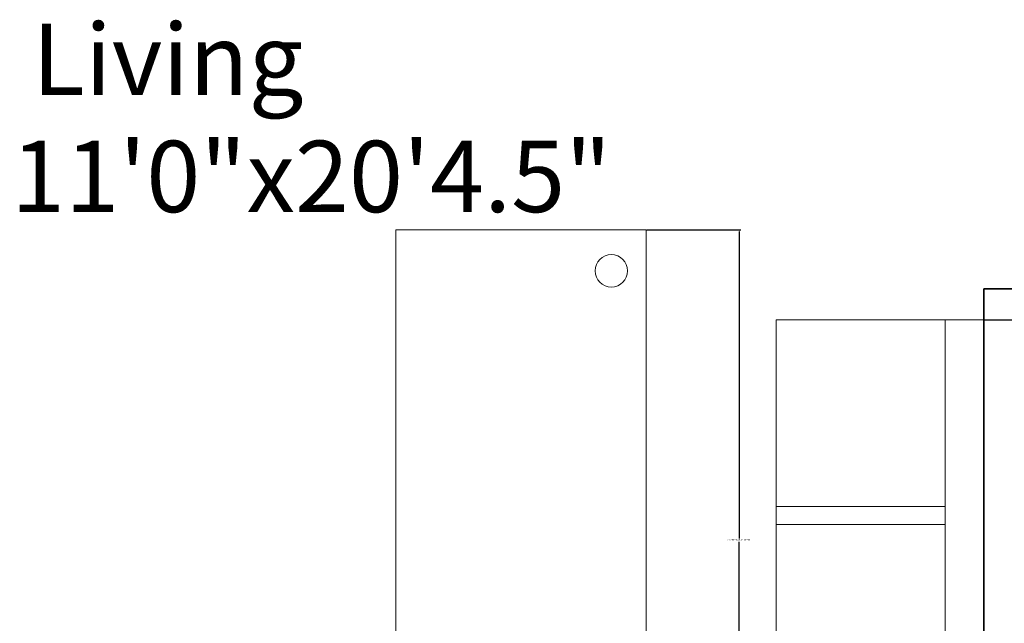
# Model space of a CAD drawing. Units: inches. Extents: x 108 to 613, y 1573 to 2319.
# Tile 7 of 11: x 325 to 434, y 2055 to 2122. Entities that reach past the tile are written whole.
import ezdxf

# ---------------------------------------------------------------- set-up
doc = ezdxf.new("R2010")
doc.units = ezdxf.units.IN
for name, color, linetype, lineweight in [('A-ANNO-DIMS', 2, 'Continuous', 18), ('A-AREA-IDEN', 3, 'Continuous', 18), ('furniture', 2, 'Continuous', 18), ('wall', 6, 'Continuous', 35)]:
    doc.layers.add(name, color=color, linetype=linetype, lineweight=lineweight)
doc.styles.get("Standard").update_dxf_attribs({"font": 'arial.ttf'})
doc.dimstyles.get("Standard").update_dxf_attribs({"dimtxt": 0.18, "dimasz": 0.18, "dimexe": 0.18, "dimexo": 0.0625, "dimgap": 0.09, "dimtad": 0, "dimtih": 1, "dimtoh": 1, "dimdec": 4, "dimzin": 0, "dimdsep": 46, "dimtxsty": 'Standard', "dimcen": 0.09, "dimadec": 0, "dimazin": 0, "dimtfac": 1, "dimtdec": 4, "dimtofl": 0, "dimtmove": 0, "dimatfit": 3, "dimfxl": 1, "dimtolj": 1, "dimtzin": 0, "dimarcsym": 0})

# ---------------------------------------------------------------- blocks, each defined once
blk = doc.blocks.new('COFFEE-TABLE')
blk.add_lwpolyline([(0, 68.46), (27.63, 68.46), (27.63, 0), (0, 0)], close=True)
for centre, radius in [((23.79, 63.93), 1.79), ((3.47, 4.05), 1.83)]:
    blk.add_circle(centre, radius)
blk = doc.blocks.new('SOFA-3-SEAT')
for p, q in [((18.7, 63.66), (18.7, 0)), ((0.03, 43.08), (18.7, 43.08)), ((0.03, 41.08), (18.7, 41.08)), ((0.03, 20.17), (18.7, 19.89)), ((0, 18.17), (18.7, 17.89))]:
    blk.add_line(p, q)
blk.add_lwpolyline([(0.03, 63.66), (22.97, 63.66), (22.97, 0), (0.03, 0)], close=True)
blk = doc.blocks.new('*D29')
at = {"layer": 'A-ANNO-DIMS', "color": 0, "lineweight": -2, "transparency": 16777216}
for p, q in [((394.08, 2098.63), (404.46, 2098.63)), ((404.28, 2098.45), (404.28, 2064.59)), ((404.28, 2030.36), (404.28, 2064.22)), ((394.08, 2030.18), (404.46, 2030.18))]:
    blk.add_line(p, q, dxfattribs=at)
at = {"layer": 'A-ANNO-DIMS', "color": 0, "transparency": 16777216}
for points in [[(404.25, 2098.45), (404.31, 2098.45), (404.28, 2098.63)], [(404.25, 2030.36), (404.31, 2030.36), (404.28, 2030.18)]]:
    blk.add_solid(points, dxfattribs=at)
at = {"layer": 'Defpoints', "color": 0, "transparency": 16777216}
for p in [(394.01, 2098.63), (404.28, 2098.63), (394.01, 2030.18)]:
    blk.add_point(p, dxfattribs=at)
at = {"layer": 'A-ANNO-DIMS', "color": 0, "transparency": 16777216, "insert": (404.28, 2064.41), "char_height": 0.18, "attachment_point": 5}
blk.add_mtext('\\A1;COFFEE TABLE 68 TYP.', dxfattribs=at)
blk = doc.blocks.new('*D31')
at = {"layer": 'A-ANNO-DIMS', "color": 0, "lineweight": -2, "transparency": 16777216}
for p, q in [((431.34, 2088.69), (441, 2088.69)), ((440.82, 2088.51), (440.82, 2057.05)), ((440.82, 2025.21), (440.82, 2056.68)), ((431.34, 2025.03), (441, 2025.03))]:
    blk.add_line(p, q, dxfattribs=at)
at = {"layer": 'A-ANNO-DIMS', "color": 0, "transparency": 16777216}
for points in [[(440.79, 2088.51), (440.85, 2088.51), (440.82, 2088.69)], [(440.79, 2025.21), (440.85, 2025.21), (440.82, 2025.03)]]:
    blk.add_solid(points, dxfattribs=at)
at = {"layer": 'Defpoints', "color": 0, "transparency": 16777216}
for p in [(431.28, 2088.69), (440.82, 2088.69), (431.28, 2025.03)]:
    blk.add_point(p, dxfattribs=at)
at = {"layer": 'A-ANNO-DIMS', "color": 0, "transparency": 16777216, "insert": (440.82, 2056.86), "char_height": 0.18, "attachment_point": 5}
blk.add_mtext('\\A1;3-SEAT SOFA 64 TYP.', dxfattribs=at)

msp = doc.modelspace()

# ---------------------------------------------------------------- linework, layer by layer
at = {"layer": 'wall'}
for q in [(435.7753, 2092.1125), (431.2753, 1997.6125)]:
    msp.add_line((431.2753, 2092.1125), q, dxfattribs=at)

# ---------------------------------------------------------------- block references
at = {"layer": 'furniture'}
for name, p in [('COFFEE-TABLE', (366.385, 2030.176)), ('SOFA-3-SEAT', (408.31, 2025.033))]:
    msp.add_blockref(name, p, dxfattribs=at)

# ---------------------------------------------------------------- texts
at = {"layer": 'A-AREA-IDEN'}
for s, height, p in [('Living', 7.87346, (326.2616, 2113.4914)), ('11\'0"x20\'4.5"', 7.873465, (323.9532, 2100.5856))]:
    msp.add_text(s, height=height, dxfattribs=at).set_placement(p)

# ---------------------------------------------------------------- dimensions: what is measured, and where the dimension line sits
at = {"layer": 'A-ANNO-DIMS'}
for base, p1, p2, text, picture, middle in [((404.2835, 2098.634), (394.0149, 2030.176), (394.0149, 2098.634), 'COFFEE TABLE <> TYP.', '*D29', (404.2835, 2064.405)), ((440.8243, 2088.6925), (431.2753, 2025.0326), (431.2753, 2088.6925), '3-SEAT SOFA <> TYP.', '*D31', (440.8243, 2056.8625))]:
    dim = msp.add_linear_dim(base=base, p1=p1, p2=p2, angle=90, text=text, dimstyle='Standard', override={"dimdec": 0, "dimlfac": 1, "dimrnd": 0, "dimzin": 0, "dimdsep": 46, "dimlunit": 2}, dxfattribs=at)
    dim.commit()
    dim.dimension.update_dxf_attribs({"geometry": picture, "text_midpoint": middle})

doc.saveas('drawing.dxf')
